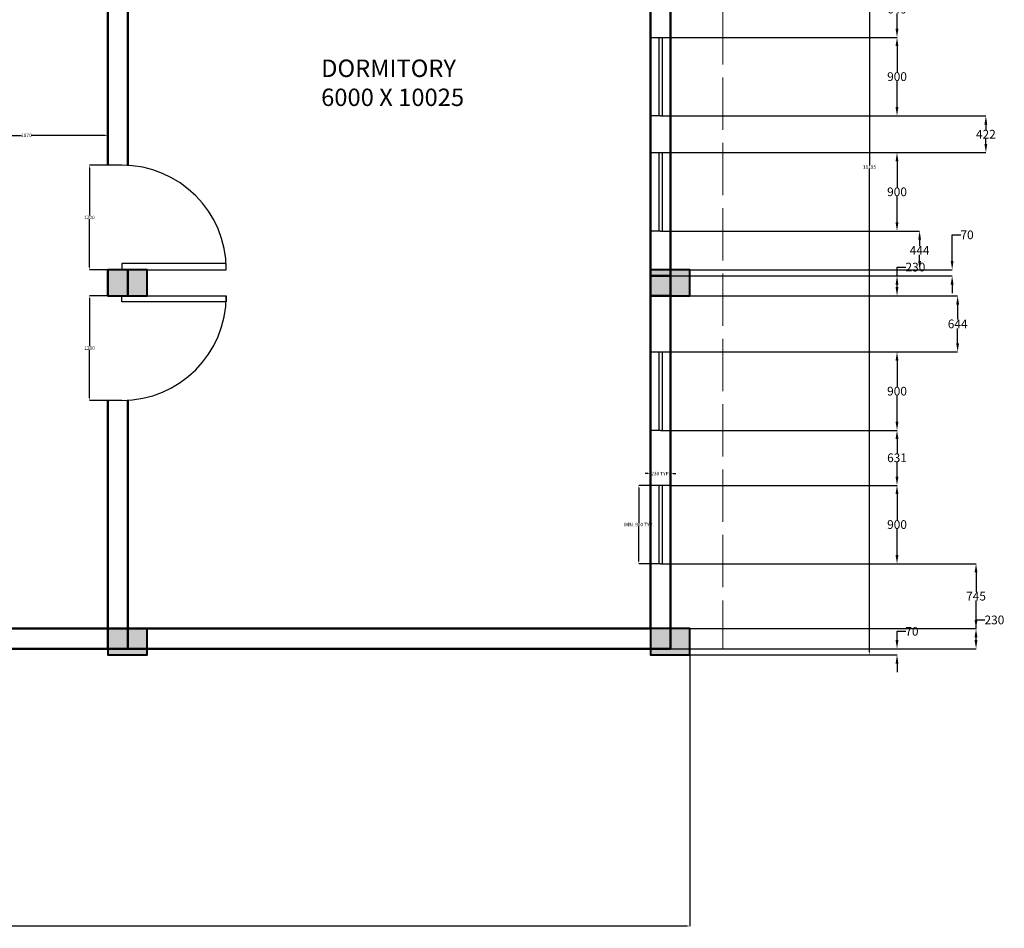
# Model space of a CAD drawing. Units: millimetres. Extents: x -17156 to 39375, y -45872 to -24892.
# Tile 10 of 12: x 5351 to 16653, y -45872 to -35444. Entities that reach past the tile are written whole.
import ezdxf

# ---------------------------------------------------------------- set-up
doc = ezdxf.new("R2010")
doc.units = ezdxf.units.MM
doc.header["$MEASUREMENT"] = 0
doc.linetypes.add('ACAD_ISO02W100', pattern=[15, 12, -3])
for name, color, linetype, lineweight in [('A-ANNO-DIMS', 2, 'Continuous', 18), ('A-AREA-IDEN', 4, 'Continuous', 25), ('A-COLS', 7, 'Continuous', 40), ('A-ROOF-OVHD', 8, 'ACAD_ISO02W100', 18), ('DOORS', 6, 'Continuous', 25), ('WALLS', 5, 'Continuous', 50), ('WINDOW', 240, 'Continuous', 25)]:
    doc.layers.add(name, color=color, linetype=linetype, lineweight=lineweight)
doc.styles.get("Standard").update_dxf_attribs({"font": 'arial.ttf'})
doc.dimstyles.get("Standard").update_dxf_attribs({"dimtxt": 40, "dimasz": 30.18, "dimexe": 0, "dimexo": 0.0625, "dimgap": 0.09, "dimtad": 0, "dimtih": 1, "dimtoh": 1, "dimdec": 0, "dimzin": 0, "dimdsep": 46, "dimtxsty": 'Standard', "dimcen": 0.09, "dimadec": 0, "dimazin": 0, "dimtfac": 1, "dimtdec": 0, "dimtofl": 0, "dimtmove": 0, "dimatfit": 3, "dimfxl": 1, "dimtolj": 1, "dimtzin": 0, "dimarcsym": 0})

# ---------------------------------------------------------------- blocks, each defined once
blk = doc.blocks.new('*U8')
for p, q in [((-750, 0), (-750, 100)), ((0, 0), (0, 100))]:
    blk.add_line(p, q)
blk.add_lwpolyline([(0, 0), (0, -750), (-43.75, -750), (-43.75, 0)], close=True)
blk.add_arc((0, 0), 750, 180, 270)
blk = doc.blocks.new('*U3')
for p, q in [((-750, 0), (-750, -100)), ((0, 0), (0, -100))]:
    blk.add_line(p, q)
blk.add_lwpolyline([(0, 0), (0, 750), (-43.75, 750), (-43.75, 0)], close=True)
blk.add_arc((0, 0), 750, 90, 180)
blk = doc.blocks.new('*D31')
at = {"layer": 'A-ANNO-DIMS', "color": 0, "lineweight": -2, "transparency": 16777216}
for p, q in [((15422, -42563), (15422, -42463)), ((15422, -42463), (15522, -42463)), ((12823, -42663), (15422, -42663)), ((13043, -42733), (15422, -42733)), ((15422, -42833), (15422, -42933))]:
    blk.add_line(p, q, dxfattribs=at)
at = {"layer": 'A-ANNO-DIMS', "color": 0, "lineweight": 100, "transparency": 16777216}
for points in [[(15405, -42563), (15438, -42563), (15422, -42663)], [(15405, -42833), (15438, -42833), (15422, -42733)]]:
    blk.add_solid(points, dxfattribs=at)
at = {"layer": 'Defpoints', "color": 0, "lineweight": 100, "transparency": 16777216}
for p in [(12823, -42663), (15422, -42663), (13043, -42733)]:
    blk.add_point(p, dxfattribs=at)
at = {"layer": 'A-ANNO-DIMS', "color": 0, "transparency": 16777216, "insert": (15593, -42463), "char_height": 100, "attachment_point": 5}
blk.add_mtext('\\A1;70', dxfattribs=at)
blk = doc.blocks.new('*D32')
at = {"layer": 'A-ANNO-DIMS', "color": 0, "lineweight": -2, "transparency": 16777216}
for p, q in [((16329, -42433), (16329, -42333)), ((16329, -42333), (16429, -42333)), ((13043, -42433), (16329, -42433)), ((16329, -42563), (16329, -42533)), ((12823, -42663), (16329, -42663))]:
    blk.add_line(p, q, dxfattribs=at)
at = {"layer": 'A-ANNO-DIMS', "color": 0, "lineweight": 100, "transparency": 16777216}
for points in [[(16312, -42533), (16345, -42533), (16329, -42433)], [(16312, -42563), (16345, -42563), (16329, -42663)]]:
    blk.add_solid(points, dxfattribs=at)
at = {"layer": 'Defpoints', "color": 0, "lineweight": 100, "transparency": 16777216}
for p in [(13043, -42433), (16329, -42433), (12823, -42663)]:
    blk.add_point(p, dxfattribs=at)
at = {"layer": 'A-ANNO-DIMS', "color": 0, "transparency": 16777216, "insert": (16540, -42333), "char_height": 100, "attachment_point": 5}
blk.add_mtext('\\A1;230', dxfattribs=at)
blk = doc.blocks.new('*D33')
at = {"layer": 'A-ANNO-DIMS', "color": 0, "lineweight": -2, "transparency": 16777216}
for p, q in [((12823, -41688), (16329, -41688)), ((16329, -41788), (16329, -42009)), ((16329, -42333), (16329, -42111)), ((13043, -42433), (16329, -42433))]:
    blk.add_line(p, q, dxfattribs=at)
at = {"layer": 'A-ANNO-DIMS', "color": 0, "lineweight": 100, "transparency": 16777216}
for points in [[(16312, -41788), (16345, -41788), (16329, -41688)], [(16312, -42333), (16345, -42333), (16329, -42433)]]:
    blk.add_solid(points, dxfattribs=at)
at = {"layer": 'Defpoints', "color": 0, "lineweight": 100, "transparency": 16777216}
for p in [(12823, -41688), (16329, -41688), (13043, -42433)]:
    blk.add_point(p, dxfattribs=at)
at = {"layer": 'A-ANNO-DIMS', "color": 0, "transparency": 16777216, "insert": (16329, -42060), "char_height": 100, "attachment_point": 5}
blk.add_mtext('\\A1;745', dxfattribs=at)
blk = doc.blocks.new('*D34')
at = {"layer": 'A-ANNO-DIMS', "color": 0, "lineweight": -2, "transparency": 16777216}
for p, q in [((12823, -40788), (15422, -40788)), ((15422, -40888), (15422, -41187)), ((15422, -41588), (15422, -41289)), ((12823, -41688), (15422, -41688))]:
    blk.add_line(p, q, dxfattribs=at)
at = {"layer": 'A-ANNO-DIMS', "color": 0, "lineweight": 100, "transparency": 16777216}
for points in [[(15405, -40888), (15438, -40888), (15422, -40788)], [(15405, -41588), (15438, -41588), (15422, -41688)]]:
    blk.add_solid(points, dxfattribs=at)
at = {"layer": 'Defpoints', "color": 0, "lineweight": 100, "transparency": 16777216}
for p in [(12823, -40788), (15422, -40788), (12823, -41688)]:
    blk.add_point(p, dxfattribs=at)
at = {"layer": 'A-ANNO-DIMS', "color": 0, "transparency": 16777216, "insert": (15422, -41238), "char_height": 100, "attachment_point": 5}
blk.add_mtext('\\A1;900', dxfattribs=at)
blk = doc.blocks.new('*D35')
at = {"layer": 'A-ANNO-DIMS', "color": 0, "lineweight": -2, "transparency": 16777216}
for p, q in [((12823, -40157), (15422, -40157)), ((15422, -40257), (15422, -40421)), ((15422, -40688), (15422, -40524)), ((12823, -40788), (15422, -40788))]:
    blk.add_line(p, q, dxfattribs=at)
at = {"layer": 'A-ANNO-DIMS', "color": 0, "lineweight": 100, "transparency": 16777216}
for points in [[(15405, -40257), (15438, -40257), (15422, -40157)], [(15405, -40688), (15438, -40688), (15422, -40788)]]:
    blk.add_solid(points, dxfattribs=at)
at = {"layer": 'Defpoints', "color": 0, "lineweight": 100, "transparency": 16777216}
for p in [(12823, -40157), (15422, -40157), (12823, -40788)]:
    blk.add_point(p, dxfattribs=at)
at = {"layer": 'A-ANNO-DIMS', "color": 0, "transparency": 16777216, "insert": (15422, -40472), "char_height": 100, "attachment_point": 5}
blk.add_mtext('\\A1;631', dxfattribs=at)
blk = doc.blocks.new('*D36')
at = {"layer": 'A-ANNO-DIMS', "color": 0, "lineweight": -2, "transparency": 16777216}
for p, q in [((12823, -39257), (15422, -39257)), ((15422, -39357), (15422, -39656)), ((15422, -40057), (15422, -39758)), ((12823, -40157), (15422, -40157))]:
    blk.add_line(p, q, dxfattribs=at)
at = {"layer": 'A-ANNO-DIMS', "color": 0, "lineweight": 100, "transparency": 16777216}
for points in [[(15405, -39357), (15438, -39357), (15422, -39257)], [(15405, -40057), (15438, -40057), (15422, -40157)]]:
    blk.add_solid(points, dxfattribs=at)
at = {"layer": 'Defpoints', "color": 0, "lineweight": 100, "transparency": 16777216}
for p in [(12823, -39257), (15422, -39257), (12823, -40157)]:
    blk.add_point(p, dxfattribs=at)
at = {"layer": 'A-ANNO-DIMS', "color": 0, "transparency": 16777216, "insert": (15422, -39707), "char_height": 100, "attachment_point": 5}
blk.add_mtext('\\A1;900', dxfattribs=at)
blk = doc.blocks.new('*D37')
at = {"layer": 'A-ANNO-DIMS', "color": 0, "lineweight": -2, "transparency": 16777216}
for p, q in [((13043, -38613), (16118, -38613)), ((16118, -38713), (16118, -38884)), ((16118, -39157), (16118, -38986)), ((12823, -39257), (16118, -39257))]:
    blk.add_line(p, q, dxfattribs=at)
at = {"layer": 'A-ANNO-DIMS', "color": 0, "lineweight": 100, "transparency": 16777216}
for points in [[(16101, -38713), (16134, -38713), (16118, -38613)], [(16101, -39157), (16134, -39157), (16118, -39257)]]:
    blk.add_solid(points, dxfattribs=at)
at = {"layer": 'Defpoints', "color": 0, "lineweight": 100, "transparency": 16777216}
for p in [(13043, -38613), (16118, -38613), (12823, -39257)]:
    blk.add_point(p, dxfattribs=at)
at = {"layer": 'A-ANNO-DIMS', "color": 0, "transparency": 16777216, "insert": (16118, -38935), "char_height": 100, "attachment_point": 5}
blk.add_mtext('\\A1;644', dxfattribs=at)
blk = doc.blocks.new('*D38')
at = {"layer": 'A-ANNO-DIMS', "color": 0, "lineweight": -2, "transparency": 16777216}
for p, q in [((15422, -38383), (15422, -38283)), ((15422, -38283), (15522, -38283)), ((12823, -38383), (15422, -38383)), ((15422, -38513), (15422, -38483)), ((13043, -38613), (15422, -38613))]:
    blk.add_line(p, q, dxfattribs=at)
at = {"layer": 'A-ANNO-DIMS', "color": 0, "lineweight": 100, "transparency": 16777216}
for points in [[(15405, -38483), (15438, -38483), (15422, -38383)], [(15405, -38513), (15438, -38513), (15422, -38613)]]:
    blk.add_solid(points, dxfattribs=at)
at = {"layer": 'Defpoints', "color": 0, "lineweight": 100, "transparency": 16777216}
for p in [(12823, -38383), (15422, -38383), (13043, -38613)]:
    blk.add_point(p, dxfattribs=at)
at = {"layer": 'A-ANNO-DIMS', "color": 0, "transparency": 16777216, "insert": (15633, -38283), "char_height": 100, "attachment_point": 5}
blk.add_mtext('\\A1;230', dxfattribs=at)
blk = doc.blocks.new('*D39')
at = {"layer": 'A-ANNO-DIMS', "color": 0, "lineweight": -2, "transparency": 16777216}
for p, q in [((16055, -38213), (16055, -37913)), ((16055, -37913), (16155, -37913)), ((13043, -38313), (16055, -38313)), ((12823, -38383), (16055, -38383)), ((16055, -38483), (16055, -38583))]:
    blk.add_line(p, q, dxfattribs=at)
at = {"layer": 'A-ANNO-DIMS', "color": 0, "lineweight": 100, "transparency": 16777216}
for points in [[(16038, -38213), (16071, -38213), (16055, -38313)], [(16038, -38483), (16071, -38483), (16055, -38383)]]:
    blk.add_solid(points, dxfattribs=at)
at = {"layer": 'Defpoints', "color": 0, "lineweight": 100, "transparency": 16777216}
for p in [(13043, -38313), (16055, -38313), (12823, -38383)]:
    blk.add_point(p, dxfattribs=at)
at = {"layer": 'A-ANNO-DIMS', "color": 0, "transparency": 16777216, "insert": (16226, -37913), "char_height": 100, "attachment_point": 5}
blk.add_mtext('\\A1;70', dxfattribs=at)
blk = doc.blocks.new('*D40')
at = {"layer": 'A-ANNO-DIMS', "color": 0, "lineweight": -2, "transparency": 16777216}
for p, q in [((12823, -37869), (15681, -37869)), ((15681, -37969), (15681, -38041)), ((15681, -38213), (15681, -38141)), ((13043, -38313), (15681, -38313))]:
    blk.add_line(p, q, dxfattribs=at)
at = {"layer": 'A-ANNO-DIMS', "color": 0, "lineweight": 100, "transparency": 16777216}
for points in [[(15665, -37969), (15698, -37969), (15681, -37869)], [(15665, -38213), (15698, -38213), (15681, -38313)]]:
    blk.add_solid(points, dxfattribs=at)
at = {"layer": 'Defpoints', "color": 0, "lineweight": 100, "transparency": 16777216}
for p in [(12823, -37869), (15681, -37869), (13043, -38313)]:
    blk.add_point(p, dxfattribs=at)
at = {"layer": 'A-ANNO-DIMS', "color": 0, "transparency": 16777216, "insert": (15681, -38091), "char_height": 100, "attachment_point": 5}
blk.add_mtext('\\A1;444', dxfattribs=at)
blk = doc.blocks.new('*D41')
at = {"layer": 'A-ANNO-DIMS', "color": 0, "lineweight": -2, "transparency": 16777216}
for p, q in [((12823, -36969), (15422, -36969)), ((15422, -37069), (15422, -37368)), ((15422, -37769), (15422, -37470)), ((12823, -37869), (15422, -37869))]:
    blk.add_line(p, q, dxfattribs=at)
at = {"layer": 'A-ANNO-DIMS', "color": 0, "lineweight": 100, "transparency": 16777216}
for points in [[(15405, -37069), (15438, -37069), (15422, -36969)], [(15405, -37769), (15438, -37769), (15422, -37869)]]:
    blk.add_solid(points, dxfattribs=at)
at = {"layer": 'Defpoints', "color": 0, "lineweight": 100, "transparency": 16777216}
for p in [(12823, -36969), (15422, -36969), (12823, -37869)]:
    blk.add_point(p, dxfattribs=at)
at = {"layer": 'A-ANNO-DIMS', "color": 0, "transparency": 16777216, "insert": (15422, -37419), "char_height": 100, "attachment_point": 5}
blk.add_mtext('\\A1;900', dxfattribs=at)
blk = doc.blocks.new('*D42')
at = {"layer": 'A-ANNO-DIMS', "color": 0, "lineweight": -2, "transparency": 16777216}
for p, q in [((12823, -36547), (16442, -36547)), ((16442, -36647), (16442, -36708)), ((16442, -36869), (16442, -36808)), ((12823, -36969), (16442, -36969))]:
    blk.add_line(p, q, dxfattribs=at)
at = {"layer": 'A-ANNO-DIMS', "color": 0, "lineweight": 100, "transparency": 16777216}
for points in [[(16425, -36647), (16458, -36647), (16442, -36547)], [(16425, -36869), (16458, -36869), (16442, -36969)]]:
    blk.add_solid(points, dxfattribs=at)
at = {"layer": 'Defpoints', "color": 0, "lineweight": 100, "transparency": 16777216}
for p in [(12823, -36547), (16442, -36547), (12823, -36969)]:
    blk.add_point(p, dxfattribs=at)
at = {"layer": 'A-ANNO-DIMS', "color": 0, "transparency": 16777216, "insert": (16442, -36758), "char_height": 100, "attachment_point": 5}
blk.add_mtext('\\A1;422', dxfattribs=at)
blk = doc.blocks.new('*D43')
at = {"layer": 'A-ANNO-DIMS', "color": 0, "lineweight": -2, "transparency": 16777216}
for p, q in [((12823, -35647), (15422, -35647)), ((15422, -35747), (15422, -36046)), ((15422, -36447), (15422, -36148)), ((12823, -36547), (15422, -36547))]:
    blk.add_line(p, q, dxfattribs=at)
at = {"layer": 'A-ANNO-DIMS', "color": 0, "lineweight": 100, "transparency": 16777216}
for points in [[(15405, -35747), (15438, -35747), (15422, -35647)], [(15405, -36447), (15438, -36447), (15422, -36547)]]:
    blk.add_solid(points, dxfattribs=at)
at = {"layer": 'Defpoints', "color": 0, "lineweight": 100, "transparency": 16777216}
for p in [(12823, -35647), (15422, -35647), (12823, -36547)]:
    blk.add_point(p, dxfattribs=at)
at = {"layer": 'A-ANNO-DIMS', "color": 0, "transparency": 16777216, "insert": (15422, -36097), "char_height": 100, "attachment_point": 5}
blk.add_mtext('\\A1;900', dxfattribs=at)
blk = doc.blocks.new('*D44')
at = {"layer": 'A-ANNO-DIMS', "color": 0, "lineweight": -2, "transparency": 16777216}
for p, q in [((13043, -34998), (15422, -34998)), ((15422, -35098), (15422, -35271)), ((15422, -35547), (15422, -35374)), ((12823, -35647), (15422, -35647))]:
    blk.add_line(p, q, dxfattribs=at)
at = {"layer": 'A-ANNO-DIMS', "color": 0, "lineweight": 100, "transparency": 16777216}
for points in [[(15405, -35098), (15438, -35098), (15422, -34998)], [(15405, -35547), (15438, -35547), (15422, -35647)]]:
    blk.add_solid(points, dxfattribs=at)
at = {"layer": 'Defpoints', "color": 0, "lineweight": 100, "transparency": 16777216}
for p in [(13043, -34998), (15422, -34998), (12823, -35647)]:
    blk.add_point(p, dxfattribs=at)
at = {"layer": 'A-ANNO-DIMS', "color": 0, "transparency": 16777216, "insert": (15422, -35322), "char_height": 100, "attachment_point": 5}
blk.add_mtext('\\A1;649', dxfattribs=at)
blk = doc.blocks.new('*D108')
at = {"layer": 'A-ANNO-DIMS', "color": 0, "lineweight": -2, "transparency": 16777216}
for p, q in [((4493, -36771), (4493, -36771)), ((4523, -36771), (5370, -36771)), ((6332, -36771), (5486, -36771)), ((6363, -36771), (6363, -36771))]:
    blk.add_line(p, q, dxfattribs=at)
at = {"layer": 'A-ANNO-DIMS', "color": 0, "lineweight": 100, "transparency": 16777216}
for points in [[(4523, -36766), (4523, -36776), (4493, -36771)], [(6332, -36766), (6332, -36776), (6363, -36771)]]:
    blk.add_solid(points, dxfattribs=at)
at = {"layer": 'Defpoints', "color": 0, "lineweight": 100, "transparency": 16777216}
for p in [(4493, -36771), (6363, -36771), (6363, -36771)]:
    blk.add_point(p, dxfattribs=at)
at = {"layer": 'A-ANNO-DIMS', "color": 0, "transparency": 16777216, "insert": (5428, -36771), "char_height": 40, "attachment_point": 5}
blk.add_mtext('\\A1;1870', dxfattribs=at)
blk = doc.blocks.new('*D114')
at = {"layer": 'A-ANNO-DIMS', "color": 0, "lineweight": -2, "transparency": 16777216}
for p, q in [((6363, -37113), (6151, -37113)), ((6151, -37143), (6151, -37692)), ((6151, -38283), (6151, -37733)), ((6363, -38313), (6151, -38313))]:
    blk.add_line(p, q, dxfattribs=at)
at = {"layer": 'A-ANNO-DIMS', "color": 0, "lineweight": 100, "transparency": 16777216}
for points in [[(6146, -37143), (6156, -37143), (6151, -37113)], [(6146, -38283), (6156, -38283), (6151, -38313)]]:
    blk.add_solid(points, dxfattribs=at)
at = {"layer": 'Defpoints', "color": 0, "lineweight": 100, "transparency": 16777216}
for p in [(6363, -37113), (6151, -38313), (6363, -38313)]:
    blk.add_point(p, dxfattribs=at)
at = {"layer": 'A-ANNO-DIMS', "color": 0, "transparency": 16777216, "insert": (6151, -37713), "char_height": 40, "attachment_point": 5}
blk.add_mtext('\\A1;1200', dxfattribs=at)
blk = doc.blocks.new('*D115')
at = {"layer": 'A-ANNO-DIMS', "color": 0, "lineweight": -2, "transparency": 16777216}
for p, q in [((6363, -38613), (6152, -38613)), ((6152, -38643), (6152, -39192)), ((6152, -39783), (6152, -39233)), ((6363, -39813), (6152, -39813))]:
    blk.add_line(p, q, dxfattribs=at)
at = {"layer": 'A-ANNO-DIMS', "color": 0, "lineweight": 100, "transparency": 16777216}
for points in [[(6147, -38643), (6157, -38643), (6152, -38613)], [(6147, -39783), (6157, -39783), (6152, -39813)]]:
    blk.add_solid(points, dxfattribs=at)
at = {"layer": 'Defpoints', "color": 0, "lineweight": 100, "transparency": 16777216}
for p in [(6363, -38613), (6152, -39813), (6363, -39813)]:
    blk.add_point(p, dxfattribs=at)
at = {"layer": 'A-ANNO-DIMS', "color": 0, "transparency": 16777216, "insert": (6152, -39213), "char_height": 40, "attachment_point": 5}
blk.add_mtext('\\A1;1200', dxfattribs=at)
blk = doc.blocks.new('WIN-900x230')
for p, q in [((0, 900), (230, 900)), ((95, 900), (95, 0)), ((135, 900), (135, 0)), ((115, 0), (0, 0)), ((115, 0), (230, 0))]:
    blk.add_line(p, q)
blk = doc.blocks.new('COL-450x300')
h = blk.add_hatch(color=256)
h.dxf.hatch_style = 1
h.paths.add_polyline_path([(0, 300), (0, 0), (450, 0), (450, 300)])
blk.add_lwpolyline([(0, 300), (0, 0), (450, 0), (450, 300)], close=True)
blk = doc.blocks.new('*D142')
at = {"layer": 'A-ANNO-DIMS', "color": 0, "lineweight": -2, "transparency": 16777216}
for p, q in [((12593, -40788), (12458, -40788)), ((12458, -40818), (12458, -41217)), ((12458, -41658), (12458, -41258)), ((12593, -41688), (12458, -41688))]:
    blk.add_line(p, q, dxfattribs=at)
at = {"layer": 'A-ANNO-DIMS', "color": 0, "lineweight": 100, "transparency": 16777216}
for points in [[(12453, -40818), (12463, -40818), (12458, -40788)], [(12453, -41658), (12463, -41658), (12458, -41688)]]:
    blk.add_solid(points, dxfattribs=at)
at = {"layer": 'Defpoints', "color": 0, "lineweight": 100, "transparency": 16777216}
for p in [(12458, -40788), (12593, -40788), (12593, -41688)]:
    blk.add_point(p, dxfattribs=at)
at = {"layer": 'A-ANNO-DIMS', "color": 0, "transparency": 16777216, "insert": (12458, -41238), "char_height": 40, "attachment_point": 5}
blk.add_mtext('\\A1;WIN. 900 TYP.', dxfattribs=at)
blk = doc.blocks.new('*D143')
at = {"layer": 'A-ANNO-DIMS', "color": 0, "lineweight": -2, "transparency": 16777216}
for p, q in [((12562, -40653), (12532, -40653)), ((12593, -40788), (12593, -40653)), ((12823, -40788), (12823, -40653)), ((12853, -40653), (12883, -40653))]:
    blk.add_line(p, q, dxfattribs=at)
at = {"layer": 'A-ANNO-DIMS', "color": 0, "lineweight": 100, "transparency": 16777216}
for points in [[(12562, -40648), (12562, -40658), (12593, -40653)], [(12853, -40648), (12853, -40658), (12823, -40653)]]:
    blk.add_solid(points, dxfattribs=at)
at = {"layer": 'Defpoints', "color": 0, "lineweight": 100, "transparency": 16777216}
for p in [(12823, -40653), (12593, -40788), (12823, -40788)]:
    blk.add_point(p, dxfattribs=at)
at = {"layer": 'A-ANNO-DIMS', "color": 0, "transparency": 16777216, "insert": (12708, -40653), "char_height": 40, "attachment_point": 5}
blk.add_mtext('\\A1;230 TYP.', dxfattribs=at)
blk = doc.blocks.new('*D146')
at = {"layer": 'A-ANNO-DIMS', "color": 0, "lineweight": -2, "transparency": 16777216}
for p, q in [((-14867, -42733), (-14867, -45846)), ((13043, -42733), (13043, -45846)), ((-14837, -45846), (-988, -45846)), ((13012, -45846), (-837, -45846))]:
    blk.add_line(p, q, dxfattribs=at)
at = {"layer": 'A-ANNO-DIMS', "color": 0, "lineweight": 100, "transparency": 16777216}
for points in [[(-14837, -45841), (-14837, -45851), (-14867, -45846)], [(13012, -45841), (13012, -45851), (13043, -45846)]]:
    blk.add_solid(points, dxfattribs=at)
at = {"layer": 'Defpoints', "color": 0, "lineweight": 100, "transparency": 16777216}
for p in [(-14867, -42733), (13043, -42733), (13043, -45846)]:
    blk.add_point(p, dxfattribs=at)
at = {"layer": 'A-ANNO-DIMS', "color": 0, "transparency": 16777216, "insert": (-912, -45846), "char_height": 40, "attachment_point": 5}
blk.add_mtext('\\A1;27910', dxfattribs=at)
blk = doc.blocks.new('*D147')
at = {"layer": 'A-ANNO-DIMS', "color": 0, "lineweight": -2, "transparency": 16777216}
for p, q in [((13043, -31538), (15106, -31538)), ((15106, -31568), (15106, -37115)), ((15106, -42703), (15106, -37156)), ((13043, -42733), (15106, -42733))]:
    blk.add_line(p, q, dxfattribs=at)
at = {"layer": 'A-ANNO-DIMS', "color": 0, "lineweight": 100, "transparency": 16777216}
for points in [[(15101, -31568), (15111, -31568), (15106, -31538)], [(15101, -42703), (15111, -42703), (15106, -42733)]]:
    blk.add_solid(points, dxfattribs=at)
at = {"layer": 'Defpoints', "color": 0, "lineweight": 100, "transparency": 16777216}
for p in [(13043, -31538), (15106, -31538), (13043, -42733)]:
    blk.add_point(p, dxfattribs=at)
at = {"layer": 'A-ANNO-DIMS', "color": 0, "transparency": 16777216, "insert": (15106, -37135), "char_height": 40, "attachment_point": 5}
blk.add_mtext('\\A1;11195', dxfattribs=at)

msp = doc.modelspace()

# ---------------------------------------------------------------- linework, layer by layer
at = {"layer": 'A-ROOF-OVHD', "ltscale": 50}
msp.add_line((13422.65, -31607.85), (13422.65, -42662.85), dxfattribs=at)
at = {"layer": 'WALLS'}
for p, q in [((12822.65, -31607.85), (12822.65, -42662.85)), ((12592.65, -31837.85), (12592.65, -42432.85)), ((6362.65, -34697.85), (6362.65, -37112.85)), ((6592.65, -34697.85), (6592.65, -37114.89)), ((6362.65, -38312.85), (6362.65, -38612.85)), ((6592.65, -38312.85), (6592.65, -38612.85)), ((12822.65, -38382.85), (12592.65, -38382.85)), ((12822.65, -38612.85), (12592.65, -38612.85)), ((6362.65, -39812.85), (6362.65, -42662.85)), ((6592.65, -39810.8), (6592.65, -42662.85)), ((12592.65, -42432.85), (-10997.35, -42432.85)), ((12822.65, -42662.85), (-14797.35, -42662.85))]:
    msp.add_line(p, q, dxfattribs=at)

# ---------------------------------------------------------------- block references
at = {"layer": 'A-COLS'}
for p in [(6362.65, -38612.85), (12592.65, -38612.85), (6362.65, -42732.85), (12592.65, -42732.85), (12592.65, -42732.85)]:
    msp.add_blockref('COL-450x300', p, dxfattribs=at)
at = {"layer": 'DOORS', "xscale": 1.6, "yscale": 1.6, "zscale": 1.6}
for name, p, rotation in [('*U3', (6522.65, -38312.85), 270), ('*U8', (6522.65, -38612.85), 90)]:
    msp.add_blockref(name, p, dxfattribs=dict(at, rotation=rotation))
at = {"layer": 'WINDOW'}
for p in [(12592.65, -36546.91), (12592.65, -37869.33), (12592.65, -40156.93), (12592.65, -41687.76)]:
    msp.add_blockref('WIN-900x230', p, dxfattribs=at)

# ---------------------------------------------------------------- texts
at = {"layer": 'A-AREA-IDEN', "insert": (8811.11, -35901.1), "char_height": 200, "attachment_point": 1}
msp.add_mtext_dynamic_manual_height_columns('{DORMITORY\\P6000 X 10025}', width=1896.3428, gutter_width=1, heights=[0], dxfattribs=at)

# ---------------------------------------------------------------- dimensions: what is measured, and where the dimension line sits
at = {"layer": 'A-ANNO-DIMS'}
for base, p1, p2, angle, override, picture, middle in [((15105.65, -31537.85), (13042.65, -42732.85), (13042.65, -31537.85), 90, {"dimdec": 0, "dimlfac": 1, "dimrnd": 0, "dimzin": 0, "dimdsep": 46, "dimlunit": 2}, '*D147', (15105.65, -37135.35)), ((15421.51, -34997.85), (12822.65, -35646.91), (13042.65, -34997.85), 270, {"dimtxt": 100, "dimasz": 100, "dimclrd": 0, "dimclre": 0, "dimclrt": 0}, '*D44', (15421.51, -35322.38)), ((15421.51, -35646.91), (12822.65, -36546.91), (12822.65, -35646.91), 270, {"dimtxt": 100, "dimasz": 100, "dimclrd": 0, "dimclre": 0, "dimclrt": 0}, '*D43', (15421.51, -36096.91)), ((16441.67, -36546.91), (12822.65, -36969.33), (12822.65, -36546.91), 270, {"dimtxt": 100, "dimasz": 100, "dimclrd": 0, "dimclre": 0, "dimclrt": 0}, '*D42', (16441.67, -36758.12)), ((15421.51, -36969.33), (12822.65, -37869.33), (12822.65, -36969.33), 270, {"dimtxt": 100, "dimasz": 100, "dimclrd": 0, "dimclre": 0, "dimclrt": 0}, '*D41', (15421.51, -37419.33)), ((6151.32, -38312.85), (6362.65, -37112.85), (6362.65, -38312.85), 90, {"dimclrd": 0, "dimclre": 0, "dimclrt": 0}, '*D114', (6151.32, -37712.85)), ((15681.31, -37869.33), (13042.65, -38312.85), (12822.65, -37869.33), 270, {"dimtxt": 100, "dimasz": 100, "dimclrd": 0, "dimclre": 0, "dimclrt": 0}, '*D40', (15681.31, -38091.09)), ((15421.51, -38382.85), (13042.65, -38612.85), (12822.65, -38382.85), 270, {"dimtxt": 100, "dimasz": 100, "dimclrd": 0, "dimclre": 0, "dimclrt": 0}, '*D38', (15632.75, -38282.85)), ((6152.12, -39812.85), (6362.65, -38612.85), (6362.65, -39812.85), 90, {"dimclrd": 0, "dimclre": 0, "dimclrt": 0}, '*D115', (6152.12, -39212.85)), ((15421.51, -39256.93), (12822.65, -40156.93), (12822.65, -39256.93), 270, {"dimtxt": 100, "dimasz": 100, "dimclrd": 0, "dimclre": 0, "dimclrt": 0}, '*D36', (15421.51, -39706.93)), ((15421.51, -40156.93), (12822.65, -40787.76), (12822.65, -40156.93), 270, {"dimtxt": 100, "dimasz": 100, "dimclrd": 0, "dimclre": 0, "dimclrt": 0}, '*D35', (15421.51, -40472.35)), ((15421.51, -40787.76), (12822.65, -41687.76), (12822.65, -40787.76), 270, {"dimtxt": 100, "dimasz": 100, "dimclrd": 0, "dimclre": 0, "dimclrt": 0}, '*D34', (15421.51, -41237.76)), ((16328.64, -41687.76), (13042.65, -42432.85), (12822.65, -41687.76), 270, {"dimtxt": 100, "dimasz": 100, "dimclrd": 0, "dimclre": 0, "dimclrt": 0}, '*D33', (16328.64, -42060.3)), ((16328.64, -42432.85), (12822.65, -42662.85), (13042.65, -42432.85), 270, {"dimtxt": 100, "dimasz": 100, "dimclrd": 0, "dimclre": 0, "dimclrt": 0}, '*D32', (16539.88, -42332.85)), ((15421.51, -42662.85), (13042.65, -42732.85), (12822.65, -42662.85), 270, {"dimtxt": 100, "dimasz": 100, "dimclrd": 0, "dimclre": 0, "dimclrt": 0}, '*D31', (15592.64, -42462.85))]:
    dim = msp.add_linear_dim(base=base, p1=p1, p2=p2, angle=angle, dimstyle='Standard', override=override, dxfattribs=at)
    dim.commit()
    dim.dimension.update_dxf_attribs({"geometry": picture, "text_midpoint": middle})
for base, p1, p2, override, picture, middle in [((6362.65, -36770.59), (4492.65, -36770.59), (6362.65, -36770.59), {"dimclrd": 0, "dimclre": 0, "dimclrt": 0}, '*D108', (5427.65, -36770.59)), ((13042.65, -45845.85), (-14867.35, -42732.85), (13042.65, -42732.85), {"dimdec": 0, "dimlfac": 1, "dimrnd": 0, "dimzin": 0, "dimdsep": 46, "dimlunit": 2}, '*D146', (-912.35, -45845.85))]:
    dim = msp.add_linear_dim(base=base, p1=p1, p2=p2, dimstyle='Standard', override=override, dxfattribs=at)
    dim.commit()
    dim.dimension.update_dxf_attribs({"geometry": picture, "text_midpoint": middle})
for base, p1, p2, picture, middle in [((16054.71, -38312.85), (12822.65, -38382.85), (13042.65, -38312.85), '*D39', (16225.84, -37912.85)), ((16117.71, -38612.85), (12822.65, -39256.93), (13042.65, -38612.85), '*D37', (16117.71, -38934.89))]:
    dim = msp.add_linear_dim(base=base, p1=p1, p2=p2, angle=270, dimstyle='Standard', override={"dimtxt": 100, "dimasz": 100, "dimclrd": 0, "dimclre": 0, "dimclrt": 0}, dxfattribs=at)
    dim.commit()
    dim.dimension.update_dxf_attribs({"geometry": picture, "text_midpoint": middle, "dimtype": 160})
dim = msp.add_linear_dim(base=(12822.65, -40652.76), p1=(12592.65, -40787.76), p2=(12822.65, -40787.76), text='<> TYP.', dimstyle='Standard', override={"dimdec": 0, "dimlfac": 1, "dimrnd": 0, "dimzin": 0, "dimdsep": 46, "dimlunit": 2}, dxfattribs=at)
dim.commit()
dim.dimension.update_dxf_attribs({"geometry": '*D143', "text_midpoint": (12707.65, -40652.76)})
dim = msp.add_linear_dim(base=(12457.65, -40787.76), p1=(12592.65, -41687.76), p2=(12592.65, -40787.76), angle=90, text='WIN. <> TYP.', dimstyle='Standard', override={"dimdec": 0, "dimlfac": 1, "dimrnd": 0, "dimzin": 0, "dimdsep": 46, "dimlunit": 2}, dxfattribs=at)
dim.commit()
dim.dimension.update_dxf_attribs({"geometry": '*D142', "text_midpoint": (12457.65, -41237.76)})

doc.saveas('drawing.dxf')
